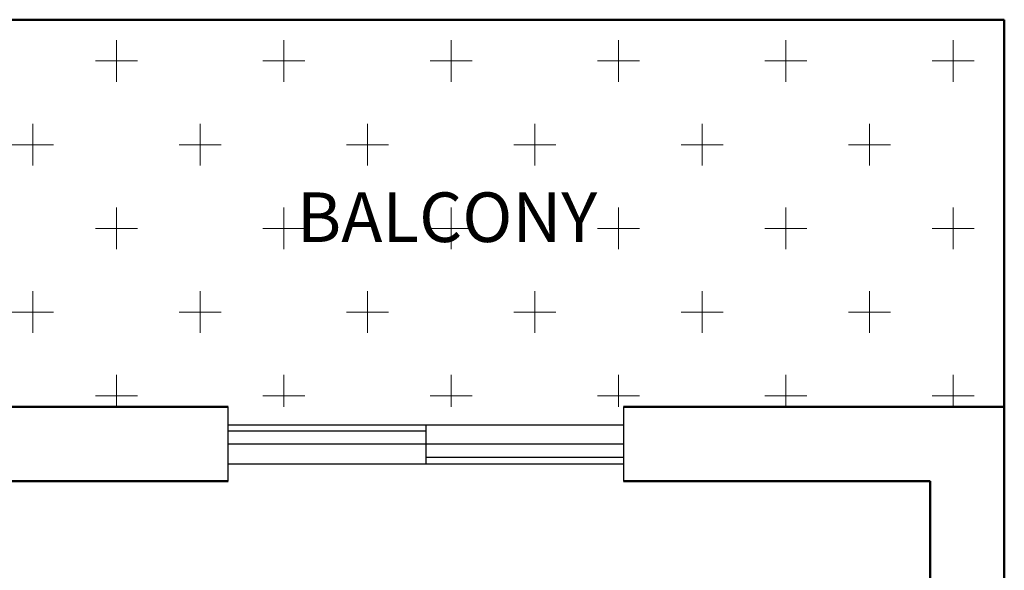
# Model space of a CAD drawing. Units: millimetres. Extents: x -857 to 54106, y -13666 to 13947.
# Tile 40 of 41: x 30856 to 33845, y 11133 to 12804. Entities that reach past the tile are written whole.
import ezdxf

# ---------------------------------------------------------------- set-up
doc = ezdxf.new("R2010")
doc.units = ezdxf.units.MM
for name, color, linetype, lineweight in [('A-AREA-IDEN', 3, 'Continuous', 18), ('A-FLOR-PATT', 252, 'Continuous', 13), ('A-GLAZ', 4, 'Continuous', 25), ('A-WALL', 7, 'Continuous', 50)]:
    doc.layers.add(name, color=color, linetype=linetype, lineweight=lineweight)
doc.styles.get("Standard").update_dxf_attribs({"font": 'arial.ttf'})

# ---------------------------------------------------------------- blocks, each defined once
blk = doc.blocks.new('WIN-1200')
for p, q in [((9371.3, 11750.2), (10571.3, 11750.2)), ((9971.3, 11750.2), (9971.3, 11630.7)), ((9371.3, 11731.7), (9971.3, 11731.7)), ((9371.3, 11691.7), (10571.3, 11691.7)), ((10571.3, 11630.7), (9371.3, 11630.7)), ((9971.3, 11651.7), (10571.3, 11651.7))]:
    blk.add_line(p, q)
for points in [[(9371.3, 11579.2), (9371.3, 11804.2)], [(10571.3, 11804.2), (10571.3, 11579.2)]]:
    blk.add_lwpolyline(points)

msp = doc.modelspace()

# ---------------------------------------------------------------- hatches: boundary and pattern name
at = {"layer": 'A-FLOR-PATT'}
h = msp.add_hatch(dxfattribs=at)
h.set_pattern_fill('CROSS', color=256, scale=40)
h.set_pattern_definition([(0, (-5489.92, -2561.3), (254, 254), [127, -381]), (90, (-5426.42, -2624.8), (-254, 254), [127, -381])])
h.paths.add_polyline_path([(33845.086, 12804.231), (30020.079, 12804.231), (30020.079, 12500.311, -0.3418929), (30695.079, 11629.231), (33845.08, 11629.231)])

# ---------------------------------------------------------------- linework, layer by layer
at = {"layer": 'A-WALL'}
for p, q in [((30020.079, 12804.231), (33845.086, 12804.231)), ((33845.086, 12804.231), (33845.08, 11629.231)), ((30020.079, 11629.231), (31489.168, 11629.231)), ((32689.168, 11629.231), (33845.08, 11629.231)), ((33845.08, 11629.231), (33845.08, 10514.82)), ((30020.079, 11404.231), (31489.168, 11404.231)), ((32689.168, 11404.231), (33620.079, 11404.231)), ((33620.079, 11404.231), (33620.079, 8154.231))]:
    msp.add_line(p, q, dxfattribs=at)

# ---------------------------------------------------------------- block references
at = {"layer": 'A-GLAZ'}
msp.add_blockref('WIN-1200', (22117.828, -175), dxfattribs=at)

# ---------------------------------------------------------------- texts
at = {"layer": 'A-AREA-IDEN', "insert": (31697.517, 12280.047), "char_height": 150.48461, "attachment_point": 1}
msp.add_mtext_dynamic_manual_height_columns('\\pxt0;BALCONY', width=2554.22693, gutter_width=18810.576, heights=[2595.835], dxfattribs=at)

doc.saveas('drawing.dxf')
